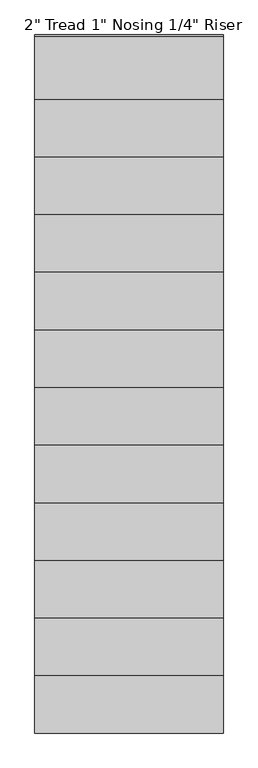
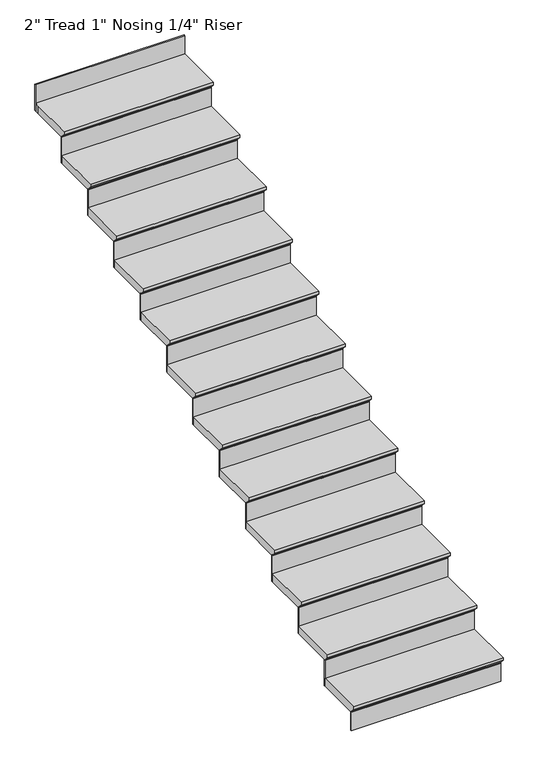
"""IFC4 building model written with IfcOpenShell, lengths in millimetres: stair flight geometry."""

from ifc_helpers import new_model, si_unit, origin, place, context, project, spatial, faceted_brep, source, transform, mapped, element, save


def stair_flight_ee9ddb45(model_context):
    return source(origin(), model_context, "Body", "Brep", [
        faceted_brep([(-2703.0415084, 19841.9216096, 40624.9005799), (-2703.0415084, 19841.9216096, 40643.9505799), (-3617.4415084, 19841.9216096, 40643.9505799), (-3617.4415084, 19841.9216096, 40624.9005799), (-2703.0415084, 19867.3216096, 40599.5005799), (-3617.4415084, 19867.3216096, 40599.5005799), (-2703.0415084, 20146.7216096, 40643.9505799), (-3617.4415084, 20146.7216096, 40643.9505799), (-3617.4415084, 19867.3216096, 40593.1505799), (-3617.4415084, 20146.7216096, 40593.1505799), (-2703.0415084, 20146.7216096, 40593.1505799), (-2703.0415084, 19867.3216096, 40593.1505799)], [[[0, 1, 2, 3]], [[4, 0, 3, 5]], [[2, 1, 6, 7]], [[8, 9, 10, 11]], [[2, 7, 9, 8, 5, 3]], [[8, 11, 4, 5]], [[6, 1, 0, 4, 11, 10]], [[7, 6, 10, 9]]]),
        faceted_brep([(-2703.0415084, 19867.3216096, 40593.1505799), (-2703.0415084, 19867.3216096, 40474.6172466), (-2703.0415084, 19873.6716096, 40474.6172466), (-2703.0415084, 19873.6716096, 40593.1505799), (-3617.4415084, 19867.3216096, 40593.1505799), (-3617.4415084, 19873.6716096, 40593.1505799), (-3617.4415084, 19873.6716096, 40474.6172466), (-3617.4415084, 19867.3216096, 40474.6172466)], [[[0, 1, 2, 3]], [[4, 5, 6, 7]], [[1, 0, 4, 7]], [[2, 1, 7, 6]], [[3, 2, 6, 5]], [[0, 3, 5, 4]]]),
        faceted_brep([(-2703.0415084, 20146.7216096, 40762.4839133), (-2703.0415084, 20146.7216096, 40593.1505799), (-2703.0415084, 20153.0716096, 40593.1505799), (-2703.0415084, 20153.0716096, 40762.4839133), (-3617.4415084, 20146.7216096, 40762.4839133), (-3617.4415084, 20153.0716096, 40762.4839133), (-3617.4415084, 20153.0716096, 40593.1505799), (-3617.4415084, 20146.7216096, 40593.1505799)], [[[0, 1, 2, 3]], [[4, 5, 6, 7]], [[1, 0, 4, 7]], [[2, 1, 7, 6]], [[3, 2, 6, 5]], [[0, 3, 5, 4]]]),
        faceted_brep([(-3617.4415084, 20121.3216096, 40813.2839133), (-2703.0415084, 20121.3216096, 40813.2839133), (-2703.0415084, 20426.1216096, 40813.2839133), (-3617.4415084, 20426.1216096, 40813.2839133), (-3617.4415084, 20146.7216096, 40762.4839133), (-3617.4415084, 20426.1216096, 40762.4839133), (-2703.0415084, 20426.1216096, 40762.4839133), (-2703.0415084, 20146.7216096, 40762.4839133), (-3617.4415084, 20146.7216096, 40768.8339133), (-3617.4415084, 20121.3216096, 40794.2339133), (-2703.0415084, 20146.7216096, 40768.8339133), (-2703.0415084, 20121.3216096, 40794.2339133)], [[[0, 1, 2, 3]], [[4, 5, 6, 7]], [[0, 3, 5, 4, 8, 9]], [[4, 7, 10, 8]], [[2, 1, 11, 10, 7, 6]], [[3, 2, 6, 5]], [[11, 1, 0, 9]], [[10, 11, 9, 8]]]),
        faceted_brep([(-2703.0415084, 20426.1216096, 40931.8172466), (-2703.0415084, 20426.1216096, 40762.4839133), (-2703.0415084, 20432.4716096, 40762.4839133), (-2703.0415084, 20432.4716096, 40931.8172466), (-3617.4415084, 20426.1216096, 40931.8172466), (-3617.4415084, 20432.4716096, 40931.8172466), (-3617.4415084, 20432.4716096, 40762.4839133), (-3617.4415084, 20426.1216096, 40762.4839133)], [[[0, 1, 2, 3]], [[4, 5, 6, 7]], [[1, 0, 4, 7]], [[2, 1, 7, 6]], [[3, 2, 6, 5]], [[0, 3, 5, 4]]]),
        faceted_brep([(-3617.4415084, 20400.7216096, 40982.6172466), (-2703.0415084, 20400.7216096, 40982.6172466), (-2703.0415084, 20705.5216096, 40982.6172466), (-3617.4415084, 20705.5216096, 40982.6172466), (-3617.4415084, 20426.1216096, 40931.8172466), (-3617.4415084, 20705.5216096, 40931.8172466), (-2703.0415084, 20705.5216096, 40931.8172466), (-2703.0415084, 20426.1216096, 40931.8172466), (-3617.4415084, 20426.1216096, 40938.1672466), (-3617.4415084, 20400.7216096, 40963.5672466), (-2703.0415084, 20426.1216096, 40938.1672466), (-2703.0415084, 20400.7216096, 40963.5672466)], [[[0, 1, 2, 3]], [[4, 5, 6, 7]], [[0, 3, 5, 4, 8, 9]], [[4, 7, 10, 8]], [[2, 1, 11, 10, 7, 6]], [[3, 2, 6, 5]], [[11, 1, 0, 9]], [[10, 11, 9, 8]]]),
        faceted_brep([(-2703.0415084, 20705.5216096, 41101.1505799), (-2703.0415084, 20705.5216096, 40931.8172466), (-2703.0415084, 20711.8716096, 40931.8172466), (-2703.0415084, 20711.8716096, 41101.1505799), (-3617.4415084, 20705.5216096, 41101.1505799), (-3617.4415084, 20711.8716096, 41101.1505799), (-3617.4415084, 20711.8716096, 40931.8172466), (-3617.4415084, 20705.5216096, 40931.8172466)], [[[0, 1, 2, 3]], [[4, 5, 6, 7]], [[1, 0, 4, 7]], [[2, 1, 7, 6]], [[3, 2, 6, 5]], [[0, 3, 5, 4]]]),
        faceted_brep([(-3617.4415084, 20680.1216096, 41151.9505799), (-2703.0415084, 20680.1216096, 41151.9505799), (-2703.0415084, 20984.9216096, 41151.9505799), (-3617.4415084, 20984.9216096, 41151.9505799), (-3617.4415084, 20705.5216096, 41101.1505799), (-3617.4415084, 20984.9216096, 41101.1505799), (-2703.0415084, 20984.9216096, 41101.1505799), (-2703.0415084, 20705.5216096, 41101.1505799), (-3617.4415084, 20705.5216096, 41107.5005799), (-3617.4415084, 20680.1216096, 41132.9005799), (-2703.0415084, 20705.5216096, 41107.5005799), (-2703.0415084, 20680.1216096, 41132.9005799)], [[[0, 1, 2, 3]], [[4, 5, 6, 7]], [[0, 3, 5, 4, 8, 9]], [[4, 7, 10, 8]], [[2, 1, 11, 10, 7, 6]], [[3, 2, 6, 5]], [[11, 1, 0, 9]], [[10, 11, 9, 8]]]),
        faceted_brep([(-2703.0415084, 20984.9216096, 41270.4839133), (-2703.0415084, 20984.9216096, 41101.1505799), (-2703.0415084, 20991.2716096, 41101.1505799), (-2703.0415084, 20991.2716096, 41270.4839133), (-3617.4415084, 20984.9216096, 41270.4839133), (-3617.4415084, 20991.2716096, 41270.4839133), (-3617.4415084, 20991.2716096, 41101.1505799), (-3617.4415084, 20984.9216096, 41101.1505799)], [[[0, 1, 2, 3]], [[4, 5, 6, 7]], [[1, 0, 4, 7]], [[2, 1, 7, 6]], [[3, 2, 6, 5]], [[0, 3, 5, 4]]]),
        faceted_brep([(-3617.4415084, 20959.5216096, 41321.2839133), (-2703.0415084, 20959.5216096, 41321.2839133), (-2703.0415084, 21264.3216096, 41321.2839133), (-3617.4415084, 21264.3216096, 41321.2839133), (-3617.4415084, 20984.9216096, 41270.4839133), (-3617.4415084, 21264.3216096, 41270.4839133), (-2703.0415084, 21264.3216096, 41270.4839133), (-2703.0415084, 20984.9216096, 41270.4839133), (-3617.4415084, 20984.9216096, 41276.8339133), (-3617.4415084, 20959.5216096, 41302.2339133), (-2703.0415084, 20984.9216096, 41276.8339133), (-2703.0415084, 20959.5216096, 41302.2339133)], [[[0, 1, 2, 3]], [[4, 5, 6, 7]], [[0, 3, 5, 4, 8, 9]], [[4, 7, 10, 8]], [[2, 1, 11, 10, 7, 6]], [[3, 2, 6, 5]], [[11, 1, 0, 9]], [[10, 11, 9, 8]]]),
        faceted_brep([(-2703.0415084, 21264.3216096, 41439.8172466), (-2703.0415084, 21264.3216096, 41270.4839133), (-2703.0415084, 21270.6716096, 41270.4839133), (-2703.0415084, 21270.6716096, 41439.8172466), (-3617.4415084, 21264.3216096, 41439.8172466), (-3617.4415084, 21270.6716096, 41439.8172466), (-3617.4415084, 21270.6716096, 41270.4839133), (-3617.4415084, 21264.3216096, 41270.4839133)], [[[0, 1, 2, 3]], [[4, 5, 6, 7]], [[1, 0, 4, 7]], [[2, 1, 7, 6]], [[3, 2, 6, 5]], [[0, 3, 5, 4]]]),
        faceted_brep([(-3617.4415084, 21238.9216096, 41490.6172466), (-2703.0415084, 21238.9216096, 41490.6172466), (-2703.0415084, 21543.7216096, 41490.6172466), (-3617.4415084, 21543.7216096, 41490.6172466), (-3617.4415084, 21264.3216096, 41439.8172466), (-3617.4415084, 21543.7216096, 41439.8172466), (-2703.0415084, 21543.7216096, 41439.8172466), (-2703.0415084, 21264.3216096, 41439.8172466), (-3617.4415084, 21264.3216096, 41446.1672466), (-3617.4415084, 21238.9216096, 41471.5672466), (-2703.0415084, 21264.3216096, 41446.1672466), (-2703.0415084, 21238.9216096, 41471.5672466)], [[[0, 1, 2, 3]], [[4, 5, 6, 7]], [[0, 3, 5, 4, 8, 9]], [[4, 7, 10, 8]], [[2, 1, 11, 10, 7, 6]], [[3, 2, 6, 5]], [[11, 1, 0, 9]], [[10, 11, 9, 8]]]),
        faceted_brep([(-2703.0415084, 21543.7216096, 41609.1505799), (-2703.0415084, 21543.7216096, 41439.8172466), (-2703.0415084, 21550.0716096, 41439.8172466), (-2703.0415084, 21550.0716096, 41609.1505799), (-3617.4415084, 21543.7216096, 41609.1505799), (-3617.4415084, 21550.0716096, 41609.1505799), (-3617.4415084, 21550.0716096, 41439.8172466), (-3617.4415084, 21543.7216096, 41439.8172466)], [[[0, 1, 2, 3]], [[4, 5, 6, 7]], [[1, 0, 4, 7]], [[2, 1, 7, 6]], [[3, 2, 6, 5]], [[0, 3, 5, 4]]]),
        faceted_brep([(-3617.4415084, 21518.3216096, 41659.9505799), (-2703.0415084, 21518.3216096, 41659.9505799), (-2703.0415084, 21823.1216096, 41659.9505799), (-3617.4415084, 21823.1216096, 41659.9505799), (-3617.4415084, 21543.7216096, 41609.1505799), (-3617.4415084, 21823.1216096, 41609.1505799), (-2703.0415084, 21823.1216096, 41609.1505799), (-2703.0415084, 21543.7216096, 41609.1505799), (-3617.4415084, 21543.7216096, 41615.5005799), (-3617.4415084, 21518.3216096, 41640.9005799), (-2703.0415084, 21543.7216096, 41615.5005799), (-2703.0415084, 21518.3216096, 41640.9005799)], [[[0, 1, 2, 3]], [[4, 5, 6, 7]], [[0, 3, 5, 4, 8, 9]], [[4, 7, 10, 8]], [[2, 1, 11, 10, 7, 6]], [[3, 2, 6, 5]], [[11, 1, 0, 9]], [[10, 11, 9, 8]]]),
        faceted_brep([(-2703.0415084, 21823.1216096, 41778.4839133), (-2703.0415084, 21823.1216096, 41609.1505799), (-2703.0415084, 21829.4716096, 41609.1505799), (-2703.0415084, 21829.4716096, 41778.4839133), (-3617.4415084, 21823.1216096, 41778.4839133), (-3617.4415084, 21829.4716096, 41778.4839133), (-3617.4415084, 21829.4716096, 41609.1505799), (-3617.4415084, 21823.1216096, 41609.1505799)], [[[0, 1, 2, 3]], [[4, 5, 6, 7]], [[1, 0, 4, 7]], [[2, 1, 7, 6]], [[3, 2, 6, 5]], [[0, 3, 5, 4]]]),
        faceted_brep([(-3617.4415084, 21797.7216096, 41829.2839133), (-2703.0415084, 21797.7216096, 41829.2839133), (-2703.0415084, 22102.5216096, 41829.2839133), (-3617.4415084, 22102.5216096, 41829.2839133), (-3617.4415084, 21823.1216096, 41778.4839133), (-3617.4415084, 22102.5216096, 41778.4839133), (-2703.0415084, 22102.5216096, 41778.4839133), (-2703.0415084, 21823.1216096, 41778.4839133), (-3617.4415084, 21823.1216096, 41784.8339133), (-3617.4415084, 21797.7216096, 41810.2339133), (-2703.0415084, 21823.1216096, 41784.8339133), (-2703.0415084, 21797.7216096, 41810.2339133)], [[[0, 1, 2, 3]], [[4, 5, 6, 7]], [[0, 3, 5, 4, 8, 9]], [[4, 7, 10, 8]], [[2, 1, 11, 10, 7, 6]], [[3, 2, 6, 5]], [[11, 1, 0, 9]], [[10, 11, 9, 8]]]),
        faceted_brep([(-2703.0415084, 22102.5216096, 41947.8172466), (-2703.0415084, 22102.5216096, 41778.4839133), (-2703.0415084, 22108.8716096, 41778.4839133), (-2703.0415084, 22108.8716096, 41947.8172466), (-3617.4415084, 22102.5216096, 41947.8172466), (-3617.4415084, 22108.8716096, 41947.8172466), (-3617.4415084, 22108.8716096, 41778.4839133), (-3617.4415084, 22102.5216096, 41778.4839133)], [[[0, 1, 2, 3]], [[4, 5, 6, 7]], [[1, 0, 4, 7]], [[2, 1, 7, 6]], [[3, 2, 6, 5]], [[0, 3, 5, 4]]]),
        faceted_brep([(-3617.4415084, 22077.1216096, 41998.6172466), (-2703.0415084, 22077.1216096, 41998.6172466), (-2703.0415084, 22381.9216096, 41998.6172466), (-3617.4415084, 22381.9216096, 41998.6172466), (-3617.4415084, 22102.5216096, 41947.8172466), (-3617.4415084, 22381.9216096, 41947.8172466), (-2703.0415084, 22381.9216096, 41947.8172466), (-2703.0415084, 22102.5216096, 41947.8172466), (-3617.4415084, 22102.5216096, 41954.1672466), (-3617.4415084, 22077.1216096, 41979.5672466), (-2703.0415084, 22102.5216096, 41954.1672466), (-2703.0415084, 22077.1216096, 41979.5672466)], [[[0, 1, 2, 3]], [[4, 5, 6, 7]], [[0, 3, 5, 4, 8, 9]], [[4, 7, 10, 8]], [[2, 1, 11, 10, 7, 6]], [[3, 2, 6, 5]], [[11, 1, 0, 9]], [[10, 11, 9, 8]]]),
        faceted_brep([(-2703.0415084, 22381.9216096, 42117.1505799), (-2703.0415084, 22381.9216096, 41947.8172466), (-2703.0415084, 22388.2716096, 41947.8172466), (-2703.0415084, 22388.2716096, 42117.1505799), (-3617.4415084, 22381.9216096, 42117.1505799), (-3617.4415084, 22388.2716096, 42117.1505799), (-3617.4415084, 22388.2716096, 41947.8172466), (-3617.4415084, 22381.9216096, 41947.8172466)], [[[0, 1, 2, 3]], [[4, 5, 6, 7]], [[1, 0, 4, 7]], [[2, 1, 7, 6]], [[3, 2, 6, 5]], [[0, 3, 5, 4]]]),
        faceted_brep([(-3617.4415084, 22356.5216096, 42167.9505799), (-2703.0415084, 22356.5216096, 42167.9505799), (-2703.0415084, 22661.3216096, 42167.9505799), (-3617.4415084, 22661.3216096, 42167.9505799), (-3617.4415084, 22381.9216096, 42117.1505799), (-3617.4415084, 22661.3216096, 42117.1505799), (-2703.0415084, 22661.3216096, 42117.1505799), (-2703.0415084, 22381.9216096, 42117.1505799), (-3617.4415084, 22381.9216096, 42123.5005799), (-3617.4415084, 22356.5216096, 42148.9005799), (-2703.0415084, 22381.9216096, 42123.5005799), (-2703.0415084, 22356.5216096, 42148.9005799)], [[[0, 1, 2, 3]], [[4, 5, 6, 7]], [[0, 3, 5, 4, 8, 9]], [[4, 7, 10, 8]], [[2, 1, 11, 10, 7, 6]], [[3, 2, 6, 5]], [[11, 1, 0, 9]], [[10, 11, 9, 8]]]),
        faceted_brep([(-2703.0415084, 22661.3216096, 42286.4839133), (-2703.0415084, 22661.3216096, 42117.1505799), (-2703.0415084, 22667.6716096, 42117.1505799), (-2703.0415084, 22667.6716096, 42286.4839133), (-3617.4415084, 22661.3216096, 42286.4839133), (-3617.4415084, 22667.6716096, 42286.4839133), (-3617.4415084, 22667.6716096, 42117.1505799), (-3617.4415084, 22661.3216096, 42117.1505799)], [[[0, 1, 2, 3]], [[4, 5, 6, 7]], [[1, 0, 4, 7]], [[2, 1, 7, 6]], [[3, 2, 6, 5]], [[0, 3, 5, 4]]]),
        faceted_brep([(-3617.4415084, 22635.9216096, 42337.2839133), (-2703.0415084, 22635.9216096, 42337.2839133), (-2703.0415084, 22940.7216096, 42337.2839133), (-3617.4415084, 22940.7216096, 42337.2839133), (-3617.4415084, 22661.3216096, 42286.4839133), (-3617.4415084, 22940.7216096, 42286.4839133), (-2703.0415084, 22940.7216096, 42286.4839133), (-2703.0415084, 22661.3216096, 42286.4839133), (-3617.4415084, 22661.3216096, 42292.8339133), (-3617.4415084, 22635.9216096, 42318.2339133), (-2703.0415084, 22661.3216096, 42292.8339133), (-2703.0415084, 22635.9216096, 42318.2339133)], [[[0, 1, 2, 3]], [[4, 5, 6, 7]], [[0, 3, 5, 4, 8, 9]], [[4, 7, 10, 8]], [[2, 1, 11, 10, 7, 6]], [[3, 2, 6, 5]], [[11, 1, 0, 9]], [[10, 11, 9, 8]]]),
        faceted_brep([(-2703.0415084, 23220.1216096, 42625.1505799), (-2703.0415084, 23220.1216096, 42455.8172466), (-2703.0415084, 23226.4716096, 42455.8172466), (-2703.0415084, 23226.4716096, 42625.1505799), (-3617.4415084, 23220.1216096, 42625.1505799), (-3617.4415084, 23226.4716096, 42625.1505799), (-3617.4415084, 23226.4716096, 42455.8172466), (-3617.4415084, 23220.1216096, 42455.8172466)], [[[0, 1, 2, 3]], [[4, 5, 6, 7]], [[1, 0, 4, 7]], [[2, 1, 7, 6]], [[3, 2, 6, 5]], [[0, 3, 5, 4]]]),
        faceted_brep([(-2703.0415084, 22940.7216096, 42455.8172466), (-2703.0415084, 22940.7216096, 42286.4839133), (-2703.0415084, 22947.0716096, 42286.4839133), (-2703.0415084, 22947.0716096, 42455.8172466), (-3617.4415084, 22940.7216096, 42455.8172466), (-3617.4415084, 22947.0716096, 42455.8172466), (-3617.4415084, 22947.0716096, 42286.4839133), (-3617.4415084, 22940.7216096, 42286.4839133)], [[[0, 1, 2, 3]], [[4, 5, 6, 7]], [[1, 0, 4, 7]], [[2, 1, 7, 6]], [[3, 2, 6, 5]], [[0, 3, 5, 4]]]),
        faceted_brep([(-3617.4415084, 23220.1216096, 42506.6172466), (-3617.4415084, 23194.7216096, 42506.6172466), (-3617.4415084, 22915.3216096, 42506.6172466), (-2703.0415084, 22915.3216096, 42506.6172466), (-2703.0415084, 23220.1216096, 42506.6172466), (-3617.4415084, 23194.7216096, 42455.8172466), (-3617.4415084, 23220.1216096, 42455.8172466), (-2703.0415084, 23220.1216096, 42455.8172466), (-2703.0415084, 22940.7216096, 42455.8172466), (-3617.4415084, 22940.7216096, 42455.8172466), (-3617.4415084, 22940.7216096, 42462.1672466), (-3617.4415084, 22915.3216096, 42487.5672466), (-2703.0415084, 22940.7216096, 42462.1672466), (-2703.0415084, 22915.3216096, 42487.5672466)], [[[0, 1, 2, 3, 4]], [[5, 6, 7, 8, 9]], [[1, 0, 6, 5]], [[2, 1, 5, 9, 10, 11]], [[9, 8, 12, 10]], [[4, 3, 13, 12, 8, 7]], [[0, 4, 7, 6]], [[13, 3, 2, 11]], [[12, 13, 11, 10]]]),
    ])


if __name__ == "__main__":
    model = new_model("IFC4")
    model_context = context("Model", 3, world=origin())
    ifc_project = project(units=[si_unit("LENGTHUNIT", "METRE", prefix="MILLI")], contexts=[model_context])
    site = spatial("IfcSite", under=ifc_project)
    building = spatial("IfcBuilding", under=site)
    placement = place(None, origin())
    stair_flight_shape = stair_flight_ee9ddb45(model_context)
    element("IfcStairFlight", 1, ObjectType="2\" Tread 1\" Nosing 1/4\" Riser", at=placement, inside=building, context=model_context, shape_type="MappedRepresentation", body=[
        mapped(stair_flight_shape, transform((0.0, 0.0, 0.0), x_axis=(1.0, 0.0, 0.0), y_axis=(0.0, 1.0, 0.0), z_axis=(0.0, 0.0, 1.0))),
    ])
    save(model, "model.ifc")
